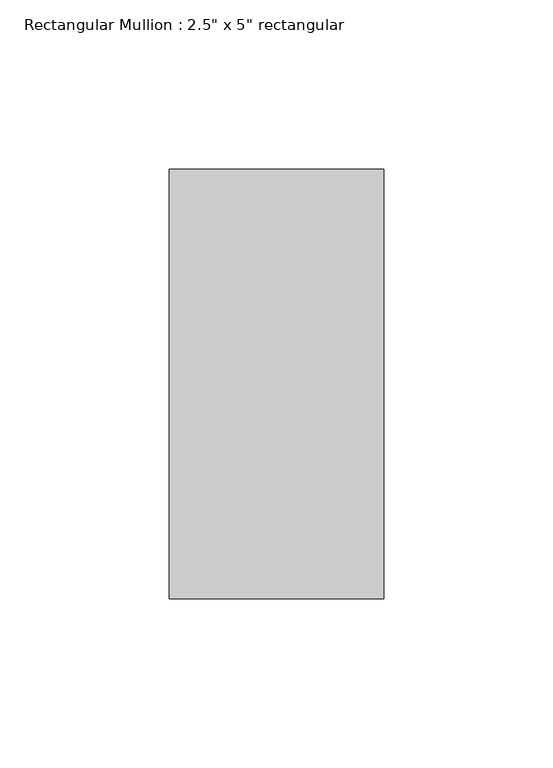
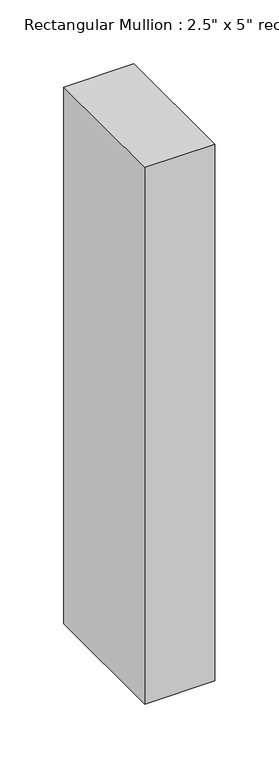
"""IFC4 building model written with IfcOpenShell, lengths in millimetres: member geometry."""

from ifc_helpers import new_model, si_unit, frame, origin, place, context, project, spatial, polyline, outline, extrude, source, transform, mapped, element, save


def member_38106158(model_context):
    return source(origin(), model_context, "Body", "SweptSolid", [
        extrude(outline(polyline([(31.75, 63.5), (31.75, -63.5), (-31.75, -63.5), (-31.75, 63.5), (31.75, 63.5)])), frame((0.0, 0.0, -513.6068067), z_axis=(0.0, 0.0, 1.0), x_axis=(1.0, 0.0, 0.0)), (0.0, 0.0, 1.0), 513.6068067),
    ])


if __name__ == "__main__":
    model = new_model("IFC4")
    model_context = context("Model", 3, world=origin())
    ifc_project = project(units=[si_unit("LENGTHUNIT", "METRE", prefix="MILLI")], contexts=[model_context])
    site = spatial("IfcSite", under=ifc_project)
    building = spatial("IfcBuilding", under=site)
    placement = place(None, origin())
    member_shape = member_38106158(model_context)
    element("IfcMember", 1, ObjectType="Rectangular Mullion : 2.5\" x 5\" rectangular", at=placement, inside=building, context=model_context, shape_type="MappedRepresentation", body=[
        mapped(member_shape, transform((0.0, 0.0, 0.0), x_axis=(1.0, 0.0, 0.0), y_axis=(0.0, 1.0, 0.0), z_axis=(0.0, 0.0, 1.0))),
    ])
    save(model, "model.ifc")

# Revit data of these elements
# Type "Rectangular Mullion : 2.5\" x 5\" rectangular"
#   built-in parameter 1007304 = 0.416667 (stored number, unit not read)
#   built-in parameter 1007301 = 0.104167 (stored number, unit not read)
#   built-in parameter 1007300 = 0.104167 (stored number, unit not read)
# Element 1 (IfcMember, "Rectangular Mullion : 2.5\" x 5\" rectangular")
#   Materials on its faces: "Aluminum"
# Materials
#   "Aluminum": class "Metal", colour RGB 247 247 247, transparency 0, Description = "Aluminum 6061", Cost = 0
